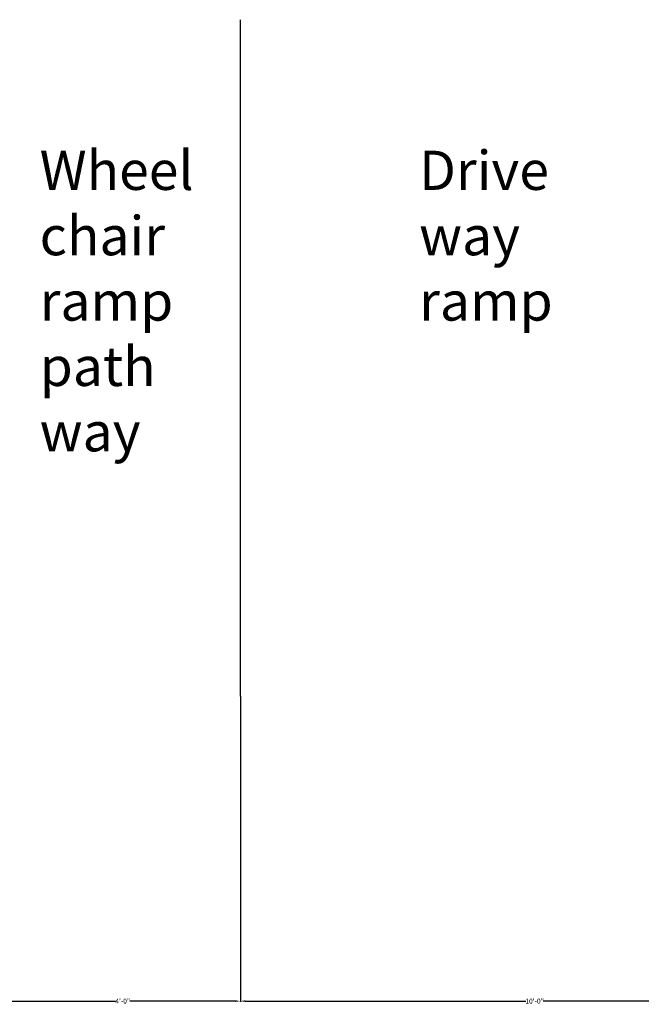
# Model space of a CAD drawing. Units: inches. Extents: x -364 to 705, y -52 to 1250.
# Tile 10 of 34: x 182 to 308, y -52 to 149. Entities that reach past the tile are written whole.
import ezdxf

# ---------------------------------------------------------------- set-up
doc = ezdxf.new("R2010")
doc.units = ezdxf.units.IN
doc.header["$MEASUREMENT"] = 0
for name, color, linetype, lineweight in [('A-ANNO-DIMS', 4, 'Continuous', 18), ('A-AREA-IDEN', 3, 'Continuous', 18), ('A-FLOR-RAMP', 7, 'Continuous', 25)]:
    doc.layers.add(name, color=color, linetype=linetype, lineweight=lineweight)
doc.styles.get("Standard").update_dxf_attribs({"font": 'arial.ttf'})
doc.dimstyles.get("Standard").update_dxf_attribs({"dimtxt": 1, "dimasz": 1, "dimexe": 0.18, "dimexo": 0.0625, "dimgap": 0.09, "dimtad": 0, "dimtih": 1, "dimtoh": 1, "dimdec": 0, "dimzin": 0, "dimdsep": 46, "dimlunit": 3, "dimtxsty": 'Standard', "dimcen": 0.09, "dimadec": 0, "dimazin": 0, "dimtfac": 1, "dimtdec": 0, "dimtofl": 0, "dimtmove": 0, "dimatfit": 3, "dimfxl": 1, "dimtolj": 1, "dimtzin": 0, "dimarcsym": 0})

# ---------------------------------------------------------------- blocks, each defined once
blk = doc.blocks.new('*D86')
at = {"layer": 'A-ANNO-DIMS', "color": 0, "lineweight": -2, "transparency": 16777216}
for p, q in [((178.58, 11.05), (178.58, -51.32)), ((226.58, 11.05), (226.58, -51.32)), ((179.58, -51.14), (201.14, -51.14)), ((225.58, -51.14), (204.02, -51.14))]:
    blk.add_line(p, q, dxfattribs=at)
at = {"layer": 'A-ANNO-DIMS', "color": 0, "transparency": 16777216}
for points in [[(179.58, -50.97), (179.58, -51.3), (178.58, -51.14)], [(225.58, -50.97), (225.58, -51.3), (226.58, -51.14)]]:
    blk.add_solid(points, dxfattribs=at)
at = {"layer": 'Defpoints', "color": 0, "transparency": 16777216}
for p in [(178.58, 11.11), (226.58, 11.11), (226.58, -51.14)]:
    blk.add_point(p, dxfattribs=at)
at = {"layer": 'A-ANNO-DIMS', "color": 0, "transparency": 16777216, "insert": (202.58, -51.14), "char_height": 1, "attachment_point": 5}
blk.add_mtext('\\A1;4\'-0"', dxfattribs=at)
blk = doc.blocks.new('*D87')
at = {"layer": 'A-ANNO-DIMS', "color": 0, "lineweight": -2, "transparency": 16777216}
for p, q in [((226.58, 11.05), (226.58, -51.32)), ((346.58, 11.05), (346.58, -51.32)), ((227.58, -51.14), (284.82, -51.14)), ((345.58, -51.14), (288.34, -51.14))]:
    blk.add_line(p, q, dxfattribs=at)
at = {"layer": 'A-ANNO-DIMS', "color": 0, "transparency": 16777216}
for points in [[(227.58, -50.97), (227.58, -51.3), (226.58, -51.14)], [(345.58, -50.97), (345.58, -51.3), (346.58, -51.14)]]:
    blk.add_solid(points, dxfattribs=at)
at = {"layer": 'Defpoints', "color": 0, "transparency": 16777216}
for p in [(226.58, 11.11), (346.58, 11.11), (346.58, -51.14)]:
    blk.add_point(p, dxfattribs=at)
at = {"layer": 'A-ANNO-DIMS', "color": 0, "transparency": 16777216, "insert": (286.58, -51.14), "char_height": 1, "attachment_point": 5}
blk.add_mtext('\\A1;10\'-0"', dxfattribs=at)

msp = doc.modelspace()

# ---------------------------------------------------------------- linework, layer by layer
at = {"layer": 'A-FLOR-RAMP'}
msp.add_line((226.58, 11.11), (226.58, 149.11), dxfattribs=at)

# ---------------------------------------------------------------- texts
at = {"layer": 'A-AREA-IDEN', "char_height": 8, "attachment_point": 1}
for s, insert in [('Wheel chair ramp path way', (185.65, 122.38)), ('Drive way ramp', (263.03, 122.38))]:
    msp.add_mtext_dynamic_manual_height_columns(s, width=30.2774, gutter_width=1, heights=[0], dxfattribs=dict(at, insert=insert))

# ---------------------------------------------------------------- dimensions: what is measured, and where the dimension line sits
at = {"layer": 'A-ANNO-DIMS'}
for base, p1, p2, picture, middle in [((226.58, -51.14), (178.58, 11.11), (226.58, 11.11), '*D86', (202.58, -51.14)), ((346.58, -51.14), (226.58, 11.11), (346.58, 11.11), '*D87', (286.58, -51.14))]:
    dim = msp.add_linear_dim(base=base, p1=p1, p2=p2, dimstyle='Standard', override={"dimdec": 1, "dimlfac": 1, "dimrnd": 0, "dimzin": 1, "dimdsep": 46, "dimlunit": 4, "dimfrac": 2}, dxfattribs=at)
    dim.commit()
    dim.dimension.update_dxf_attribs({"geometry": picture, "text_midpoint": middle})

doc.saveas('drawing.dxf')
